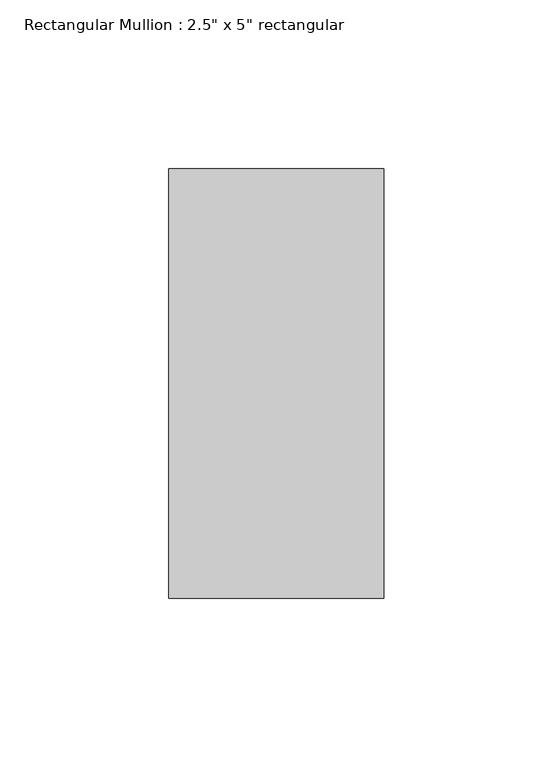
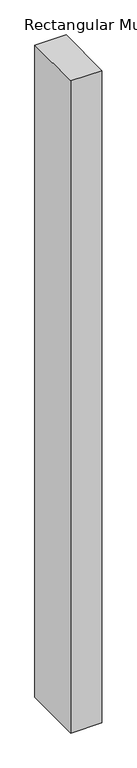
"""IFC4 building model written with IfcOpenShell, lengths in millimetres: member geometry."""

from ifc_helpers import new_model, si_unit, frame, origin, place, context, project, spatial, polyline, outline, extrude, source, transform, mapped, element, save


def member_0bf31a60(model_context):
    return source(origin(), model_context, "Body", "SweptSolid", [
        extrude(outline(polyline([(31.75, 63.5), (31.75, -63.5), (-31.75, -63.5), (-31.75, 63.5), (31.75, 63.5)])), frame((0.0, 0.0, -1408.187673), z_axis=(0.0, 0.0, 1.0), x_axis=(1.0, 0.0, 0.0)), (0.0, 0.0, 1.0), 1408.187673),
    ])


if __name__ == "__main__":
    model = new_model("IFC4")
    model_context = context("Model", 3, world=origin())
    ifc_project = project(units=[si_unit("LENGTHUNIT", "METRE", prefix="MILLI")], contexts=[model_context])
    site = spatial("IfcSite", under=ifc_project)
    building = spatial("IfcBuilding", under=site)
    placement = place(None, origin())
    member_shape = member_0bf31a60(model_context)
    element("IfcMember", 1, ObjectType="Rectangular Mullion : 2.5\" x 5\" rectangular", at=placement, inside=building, context=model_context, shape_type="MappedRepresentation", body=[
        mapped(member_shape, transform((0.0, 0.0, 0.0), x_axis=(1.0, 0.0, 0.0), y_axis=(0.0, 1.0, 0.0), z_axis=(0.0, 0.0, 1.0))),
    ])
    save(model, "model.ifc")

# Revit data of these elements
# Type "Rectangular Mullion : 2.5\" x 5\" rectangular"
#   built-in parameter 1007304 = 0.416667 (stored number, unit not read)
#   built-in parameter 1007301 = 0.104167 (stored number, unit not read)
#   built-in parameter 1007300 = 0.104167 (stored number, unit not read)
# Element 1 (IfcMember, "Rectangular Mullion : 2.5\" x 5\" rectangular")
#   Materials on its faces: "Aluminum"
# Materials
#   "Aluminum": class "Metal", colour RGB 247 247 247, transparency 0, Description = "Aluminum 6061", Cost = 0
